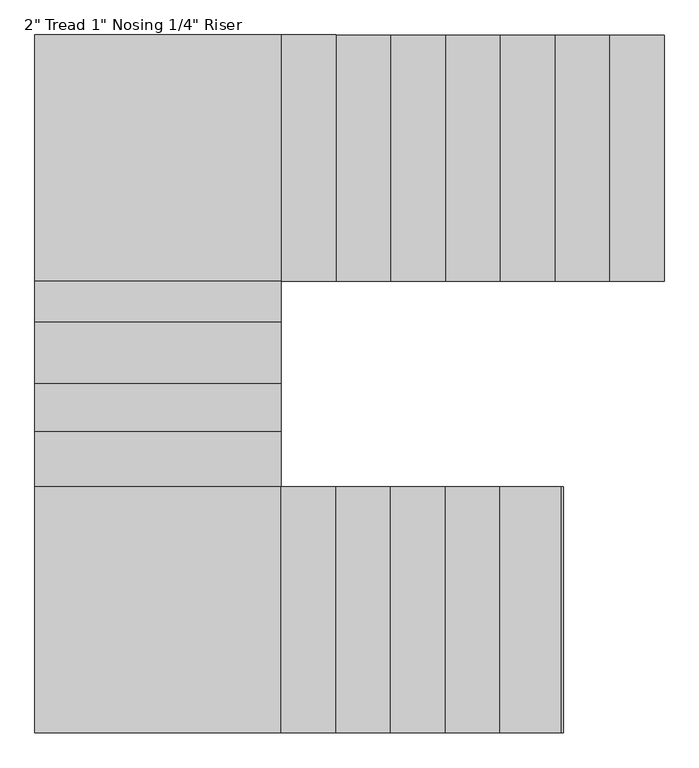
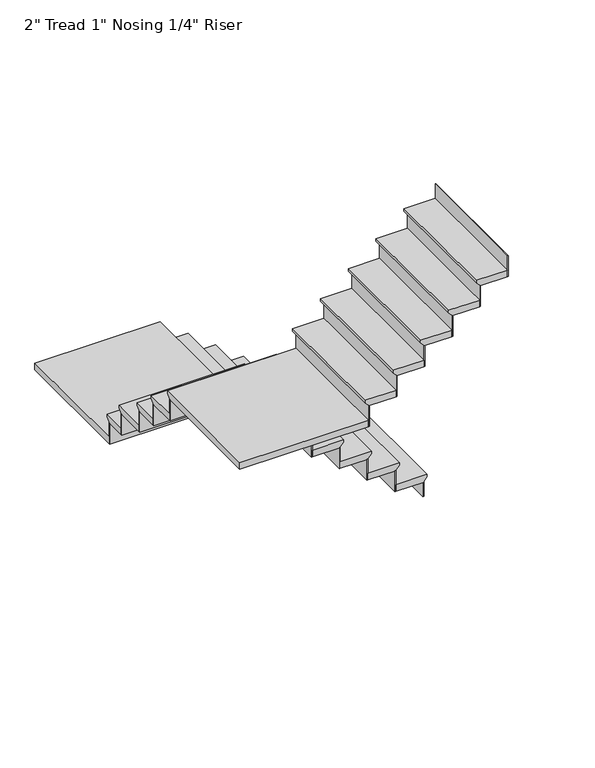
"""IFC4 building model written with IfcOpenShell, lengths in millimetres: stair flight geometry."""

from ifc_helpers import new_model, si_unit, origin, place, context, project, spatial, faceted_brep, source, transform, mapped, element, save


def stair_flight_32cec8f3(model_context):
    return source(origin(), model_context, "Body", "Brep", [
        faceted_brep([(-3603.1340247, 922.0319954, 3341.7710526), (-3603.1340247, 922.0319954, 3360.8210526), (-3603.1340247, 7.6319954, 3360.8210526), (-3603.1340247, 7.6319954, 3341.7710526), (-3628.5340247, 922.0319954, 3316.3710526), (-3628.5340247, 7.6319954, 3316.3710526), (-3831.7340247, 922.0319954, 3360.8210526), (-3831.7340247, 7.6319954, 3360.8210526), (-3628.5340247, 7.6319954, 3310.0210526), (-3831.7340247, 7.6319954, 3310.0210526), (-3831.7340247, 922.0319954, 3310.0210526), (-3628.5340247, 922.0319954, 3310.0210526)], [[[0, 1, 2, 3]], [[4, 0, 3, 5]], [[2, 1, 6, 7]], [[8, 9, 10, 11]], [[2, 7, 9, 8, 5, 3]], [[8, 11, 4, 5]], [[6, 1, 0, 4, 11, 10]], [[7, 6, 10, 9]]]),
        faceted_brep([(-3628.5340247, 922.0319954, 3310.0210526), (-3628.5340247, 922.0319954, 3200.4), (-3634.8840247, 922.0319954, 3200.4), (-3634.8840247, 922.0319954, 3310.0210526), (-3628.5340247, 7.6319954, 3310.0210526), (-3634.8840247, 7.6319954, 3310.0210526), (-3634.8840247, 7.6319954, 3200.4), (-3628.5340247, 7.6319954, 3200.4)], [[[0, 1, 2, 3]], [[4, 5, 6, 7]], [[1, 0, 4, 7]], [[2, 1, 7, 6]], [[3, 2, 6, 5]], [[0, 3, 5, 4]]]),
        faceted_brep([(-3831.7340247, 922.0319954, 3470.4421053), (-3831.7340247, 922.0319954, 3310.0210526), (-3838.0840247, 922.0319954, 3310.0210526), (-3838.0840247, 922.0319954, 3470.4421053), (-3831.7340247, 7.6319954, 3470.4421053), (-3838.0840247, 7.6319954, 3470.4421053), (-3838.0840247, 7.6319954, 3310.0210526), (-3831.7340247, 7.6319954, 3310.0210526)], [[[0, 1, 2, 3]], [[4, 5, 6, 7]], [[1, 0, 4, 7]], [[2, 1, 7, 6]], [[3, 2, 6, 5]], [[0, 3, 5, 4]]]),
        faceted_brep([(-3806.3340247, 7.6319954, 3521.2421053), (-3806.3340247, 922.0319954, 3521.2421053), (-4034.9340247, 922.0319954, 3521.2421053), (-4034.9340247, 7.6319954, 3521.2421053), (-3831.7340247, 7.6319954, 3470.4421053), (-4034.9340247, 7.6319954, 3470.4421053), (-4034.9340247, 922.0319954, 3470.4421053), (-3831.7340247, 922.0319954, 3470.4421053), (-3831.7340247, 7.6319954, 3476.7921053), (-3806.3340247, 7.6319954, 3502.1921053), (-3831.7340247, 922.0319954, 3476.7921053), (-3806.3340247, 922.0319954, 3502.1921053)], [[[0, 1, 2, 3]], [[4, 5, 6, 7]], [[0, 3, 5, 4, 8, 9]], [[4, 7, 10, 8]], [[2, 1, 11, 10, 7, 6]], [[3, 2, 6, 5]], [[11, 1, 0, 9]], [[10, 11, 9, 8]]]),
        faceted_brep([(-4034.9340247, 922.0319954, 3630.8631579), (-4034.9340247, 922.0319954, 3470.4421053), (-4041.2840247, 922.0319954, 3470.4421053), (-4041.2840247, 922.0319954, 3630.8631579), (-4034.9340247, 7.6319954, 3630.8631579), (-4041.2840247, 7.6319954, 3630.8631579), (-4041.2840247, 7.6319954, 3470.4421053), (-4034.9340247, 7.6319954, 3470.4421053)], [[[0, 1, 2, 3]], [[4, 5, 6, 7]], [[1, 0, 4, 7]], [[2, 1, 7, 6]], [[3, 2, 6, 5]], [[0, 3, 5, 4]]]),
        faceted_brep([(-4009.5340247, 7.6319954, 3681.6631579), (-4009.5340247, 922.0319954, 3681.6631579), (-4238.1340247, 922.0319954, 3681.6631579), (-4238.1340247, 7.6319954, 3681.6631579), (-4034.9340247, 7.6319954, 3630.8631579), (-4238.1340247, 7.6319954, 3630.8631579), (-4238.1340247, 922.0319954, 3630.8631579), (-4034.9340247, 922.0319954, 3630.8631579), (-4034.9340247, 7.6319954, 3637.2131579), (-4009.5340247, 7.6319954, 3662.6131579), (-4034.9340247, 922.0319954, 3637.2131579), (-4009.5340247, 922.0319954, 3662.6131579)], [[[0, 1, 2, 3]], [[4, 5, 6, 7]], [[0, 3, 5, 4, 8, 9]], [[4, 7, 10, 8]], [[2, 1, 11, 10, 7, 6]], [[3, 2, 6, 5]], [[11, 1, 0, 9]], [[10, 11, 9, 8]]]),
        faceted_brep([(-4238.1340247, 922.0319954, 3791.2842105), (-4238.1340247, 922.0319954, 3630.8631579), (-4244.4840247, 922.0319954, 3630.8631579), (-4244.4840247, 922.0319954, 3791.2842105), (-4238.1340247, 7.6319954, 3791.2842105), (-4244.4840247, 7.6319954, 3791.2842105), (-4244.4840247, 7.6319954, 3630.8631579), (-4238.1340247, 7.6319954, 3630.8631579)], [[[0, 1, 2, 3]], [[4, 5, 6, 7]], [[1, 0, 4, 7]], [[2, 1, 7, 6]], [[3, 2, 6, 5]], [[0, 3, 5, 4]]]),
        faceted_brep([(-4212.7340247, 7.6319954, 3842.0842105), (-4212.7340247, 922.0319954, 3842.0842105), (-4441.3340247, 922.0319954, 3842.0842105), (-4441.3340247, 7.6319954, 3842.0842105), (-4238.1340247, 7.6319954, 3791.2842105), (-4441.3340247, 7.6319954, 3791.2842105), (-4441.3340247, 922.0319954, 3791.2842105), (-4238.1340247, 922.0319954, 3791.2842105), (-4238.1340247, 7.6319954, 3797.6342105), (-4212.7340247, 7.6319954, 3823.0342105), (-4238.1340247, 922.0319954, 3797.6342105), (-4212.7340247, 922.0319954, 3823.0342105)], [[[0, 1, 2, 3]], [[4, 5, 6, 7]], [[0, 3, 5, 4, 8, 9]], [[4, 7, 10, 8]], [[2, 1, 11, 10, 7, 6]], [[3, 2, 6, 5]], [[11, 1, 0, 9]], [[10, 11, 9, 8]]]),
        faceted_brep([(-4441.3340247, 922.0319954, 3951.7052632), (-4441.3340247, 922.0319954, 3791.2842105), (-4447.6840247, 922.0319954, 3791.2842105), (-4447.6840247, 922.0319954, 3951.7052632), (-4441.3340247, 7.6319954, 3951.7052632), (-4447.6840247, 7.6319954, 3951.7052632), (-4447.6840247, 7.6319954, 3791.2842105), (-4441.3340247, 7.6319954, 3791.2842105)], [[[0, 1, 2, 3]], [[4, 5, 6, 7]], [[1, 0, 4, 7]], [[2, 1, 7, 6]], [[3, 2, 6, 5]], [[0, 3, 5, 4]]]),
        faceted_brep([(-4415.9340247, 7.6319954, 4002.5052632), (-4415.9340247, 922.0319954, 4002.5052632), (-4644.5340247, 922.0319954, 4002.5052632), (-4644.5340247, 7.6319954, 4002.5052632), (-4441.3340247, 7.6319954, 3951.7052632), (-4644.5340247, 7.6319954, 3951.7052632), (-4644.5340247, 922.0319954, 3951.7052632), (-4441.3340247, 922.0319954, 3951.7052632), (-4441.3340247, 7.6319954, 3958.0552632), (-4415.9340247, 7.6319954, 3983.4552632), (-4441.3340247, 922.0319954, 3958.0552632), (-4415.9340247, 922.0319954, 3983.4552632)], [[[0, 1, 2, 3]], [[4, 5, 6, 7]], [[0, 3, 5, 4, 8, 9]], [[4, 7, 10, 8]], [[2, 1, 11, 10, 7, 6]], [[3, 2, 6, 5]], [[11, 1, 0, 9]], [[10, 11, 9, 8]]]),
        faceted_brep([(-4644.5340247, 922.0319954, 4112.1263158), (-4644.5340247, 922.0319954, 3951.7052632), (-4650.8840247, 922.0319954, 3951.7052632), (-4650.8840247, 922.0319954, 4112.1263158), (-4644.5340247, 7.6319954, 4112.1263158), (-4650.8840247, 7.6319954, 4112.1263158), (-4650.8840247, 7.6319954, 3951.7052632), (-4644.5340247, 7.6319954, 3951.7052632)], [[[0, 1, 2, 3]], [[4, 5, 6, 7]], [[1, 0, 4, 7]], [[2, 1, 7, 6]], [[3, 2, 6, 5]], [[0, 3, 5, 4]]]),
        faceted_brep([(-4619.1340247, 7.6319954, 4162.9263158), (-4619.1340247, 922.0319954, 4162.9263158), (-4847.7340247, 922.0319954, 4162.9263158), (-4847.7340247, 7.6319954, 4162.9263158), (-4644.5340247, 7.6319954, 4112.1263158), (-4847.7340247, 7.6319954, 4112.1263158), (-4847.7340247, 922.0319954, 4112.1263158), (-4644.5340247, 922.0319954, 4112.1263158), (-4644.5340247, 7.6319954, 4118.4763158), (-4619.1340247, 7.6319954, 4143.8763158), (-4644.5340247, 922.0319954, 4118.4763158), (-4619.1340247, 922.0319954, 4143.8763158)], [[[0, 1, 2, 3]], [[4, 5, 6, 7]], [[0, 3, 5, 4, 8, 9]], [[4, 7, 10, 8]], [[2, 1, 11, 10, 7, 6]], [[3, 2, 6, 5]], [[11, 1, 0, 9]], [[10, 11, 9, 8]]]),
        faceted_brep([(-4847.7340247, 922.0319954, 4272.5473684), (-4847.7340247, 922.0319954, 4112.1263158), (-4854.0840247, 922.0319954, 4112.1263158), (-4854.0840247, 922.0319954, 4272.5473684), (-4847.7340247, 7.6319954, 4272.5473684), (-4854.0840247, 7.6319954, 4272.5473684), (-4854.0840247, 7.6319954, 4112.1263158), (-4847.7340247, 7.6319954, 4112.1263158)], [[[0, 1, 2, 3]], [[4, 5, 6, 7]], [[1, 0, 4, 7]], [[2, 1, 7, 6]], [[3, 2, 6, 5]], [[0, 3, 5, 4]]]),
        faceted_brep([(-4822.3340247, 7.6319954, 4323.3473684), (-4822.3340247, 922.0319954, 4323.3473684), (-5050.9340247, 922.0319954, 4323.3473684), (-5050.9340247, 7.6319954, 4323.3473684), (-4847.7340247, 7.6319954, 4272.5473684), (-5050.9340247, 7.6319954, 4272.5473684), (-5050.9340247, 922.0319954, 4272.5473684), (-4847.7340247, 922.0319954, 4272.5473684), (-4847.7340247, 7.6319954, 4278.8973684), (-4822.3340247, 7.6319954, 4304.2973684), (-4847.7340247, 922.0319954, 4278.8973684), (-4822.3340247, 922.0319954, 4304.2973684)], [[[0, 1, 2, 3]], [[4, 5, 6, 7]], [[0, 3, 5, 4, 8, 9]], [[4, 7, 10, 8]], [[2, 1, 11, 10, 7, 6]], [[3, 2, 6, 5]], [[11, 1, 0, 9]], [[10, 11, 9, 8]]]),
        faceted_brep([(-5050.9340247, 922.0319954, 4432.9684211), (-5050.9340247, 922.0319954, 4272.5473684), (-5057.2840247, 922.0319954, 4272.5473684), (-5057.2840247, 922.0319954, 4432.9684211), (-5050.9340247, 7.6319954, 4432.9684211), (-5057.2840247, 7.6319954, 4432.9684211), (-5057.2840247, 7.6319954, 4272.5473684), (-5050.9340247, 7.6319954, 4272.5473684)], [[[0, 1, 2, 3]], [[4, 5, 6, 7]], [[1, 0, 4, 7]], [[2, 1, 7, 6]], [[3, 2, 6, 5]], [[0, 3, 5, 4]]]),
        faceted_brep([(-5939.9340247, 922.0319954, 4483.7684211), (-5939.9340247, -17.7680046, 4483.7684211), (-5025.5340247, -17.7680046, 4483.7684211), (-5025.5340247, 922.0319954, 4483.7684211), (-5025.5340247, 7.6319954, 4432.9684211), (-5025.5340247, -17.7680046, 4432.9684211), (-5939.9340247, -17.7680046, 4432.9684211), (-5939.9340247, 922.0319954, 4432.9684211), (-5050.9340247, 922.0319954, 4432.9684211), (-5050.9340247, 7.6319954, 4432.9684211), (-5025.5340247, 7.6319954, 4464.7184211), (-5025.5340247, 922.0319954, 4464.7184211), (-5050.9340247, 7.6319954, 4439.3184211), (-5050.9340247, 922.0319954, 4439.3184211)], [[[0, 1, 2, 3]], [[4, 5, 6, 7, 8, 9]], [[3, 2, 5, 4, 10, 11]], [[4, 9, 12, 10]], [[9, 8, 13, 12]], [[0, 3, 11, 13, 8, 7]], [[1, 0, 7, 6]], [[2, 1, 6, 5]], [[13, 11, 10, 12]]]),
        faceted_brep([(-5939.9340247, -17.7680046, 4593.3894737), (-5939.9340247, -17.7680046, 4432.9684211), (-5939.9340247, -24.1180046, 4432.9684211), (-5939.9340247, -24.1180046, 4593.3894737), (-5025.5340247, -17.7680046, 4593.3894737), (-5025.5340247, -24.1180046, 4593.3894737), (-5025.5340247, -24.1180046, 4432.9684211), (-5025.5340247, -17.7680046, 4432.9684211)], [[[0, 1, 2, 3]], [[4, 5, 6, 7]], [[1, 0, 4, 7]], [[2, 1, 7, 6]], [[3, 2, 6, 5]], [[0, 3, 5, 4]]]),
        faceted_brep([(-5025.5340247, 7.6319954, 4644.1894737), (-5939.9340247, 7.6319954, 4644.1894737), (-5939.9340247, -170.1680046, 4644.1894737), (-5025.5340247, -170.1680046, 4644.1894737), (-5025.5340247, -17.7680046, 4593.3894737), (-5025.5340247, -170.1680046, 4593.3894737), (-5939.9340247, -170.1680046, 4593.3894737), (-5939.9340247, -17.7680046, 4593.3894737), (-5025.5340247, -17.7680046, 4599.7394737), (-5025.5340247, 7.6319954, 4625.1394737), (-5939.9340247, -17.7680046, 4599.7394737), (-5939.9340247, 7.6319954, 4625.1394737)], [[[0, 1, 2, 3]], [[4, 5, 6, 7]], [[0, 3, 5, 4, 8, 9]], [[4, 7, 10, 8]], [[2, 1, 11, 10, 7, 6]], [[3, 2, 6, 5]], [[11, 1, 0, 9]], [[10, 11, 9, 8]]]),
        faceted_brep([(-5939.9340247, -170.1680046, 4753.8105263), (-5939.9340247, -170.1680046, 4593.3894737), (-5939.9340247, -176.5180046, 4593.3894737), (-5939.9340247, -176.5180046, 4753.8105263), (-5025.5340247, -170.1680046, 4753.8105263), (-5025.5340247, -176.5180046, 4753.8105263), (-5025.5340247, -176.5180046, 4593.3894737), (-5025.5340247, -170.1680046, 4593.3894737)], [[[0, 1, 2, 3]], [[4, 5, 6, 7]], [[1, 0, 4, 7]], [[2, 1, 7, 6]], [[3, 2, 6, 5]], [[0, 3, 5, 4]]]),
        faceted_brep([(-5025.5340247, -144.7680046, 4804.6105263), (-5939.9340247, -144.7680046, 4804.6105263), (-5939.9340247, -398.7680046, 4804.6105263), (-5025.5340247, -398.7680046, 4804.6105263), (-5025.5340247, -170.1680046, 4753.8105263), (-5025.5340247, -398.7680046, 4753.8105263), (-5939.9340247, -398.7680046, 4753.8105263), (-5939.9340247, -170.1680046, 4753.8105263), (-5025.5340247, -170.1680046, 4760.1605263), (-5025.5340247, -144.7680046, 4785.5605263), (-5939.9340247, -170.1680046, 4760.1605263), (-5939.9340247, -144.7680046, 4785.5605263)], [[[0, 1, 2, 3]], [[4, 5, 6, 7]], [[0, 3, 5, 4, 8, 9]], [[4, 7, 10, 8]], [[2, 1, 11, 10, 7, 6]], [[3, 2, 6, 5]], [[11, 1, 0, 9]], [[10, 11, 9, 8]]]),
        faceted_brep([(-5939.9340247, -398.7680046, 4914.2315789), (-5939.9340247, -398.7680046, 4753.8105263), (-5939.9340247, -405.1180046, 4753.8105263), (-5939.9340247, -405.1180046, 4914.2315789), (-5025.5340247, -398.7680046, 4914.2315789), (-5025.5340247, -405.1180046, 4914.2315789), (-5025.5340247, -405.1180046, 4753.8105263), (-5025.5340247, -398.7680046, 4753.8105263)], [[[0, 1, 2, 3]], [[4, 5, 6, 7]], [[1, 0, 4, 7]], [[2, 1, 7, 6]], [[3, 2, 6, 5]], [[0, 3, 5, 4]]]),
        faceted_brep([(-5025.5340247, -373.3680046, 4965.0315789), (-5939.9340247, -373.3680046, 4965.0315789), (-5939.9340247, -576.5680046, 4965.0315789), (-5025.5340247, -576.5680046, 4965.0315789), (-5025.5340247, -398.7680046, 4914.2315789), (-5025.5340247, -576.5680046, 4914.2315789), (-5939.9340247, -576.5680046, 4914.2315789), (-5939.9340247, -398.7680046, 4914.2315789), (-5025.5340247, -398.7680046, 4920.5815789), (-5025.5340247, -373.3680046, 4945.9815789), (-5939.9340247, -398.7680046, 4920.5815789), (-5939.9340247, -373.3680046, 4945.9815789)], [[[0, 1, 2, 3]], [[4, 5, 6, 7]], [[0, 3, 5, 4, 8, 9]], [[4, 7, 10, 8]], [[2, 1, 11, 10, 7, 6]], [[3, 2, 6, 5]], [[11, 1, 0, 9]], [[10, 11, 9, 8]]]),
        faceted_brep([(-5939.9340247, -576.5680046, 5074.6526316), (-5939.9340247, -576.5680046, 4914.2315789), (-5939.9340247, -582.9180046, 4914.2315789), (-5939.9340247, -582.9180046, 5074.6526316), (-5025.5340247, -576.5680046, 5074.6526316), (-5025.5340247, -582.9180046, 5074.6526316), (-5025.5340247, -582.9180046, 4914.2315789), (-5025.5340247, -576.5680046, 4914.2315789)], [[[0, 1, 2, 3]], [[4, 5, 6, 7]], [[1, 0, 4, 7]], [[2, 1, 7, 6]], [[3, 2, 6, 5]], [[0, 3, 5, 4]]]),
        faceted_brep([(-5025.5340247, -551.1680046, 5125.4526316), (-5939.9340247, -551.1680046, 5125.4526316), (-5939.9340247, -779.7680046, 5125.4526316), (-5025.5340247, -779.7680046, 5125.4526316), (-5025.5340247, -576.5680046, 5074.6526316), (-5025.5340247, -779.7680046, 5074.6526316), (-5939.9340247, -779.7680046, 5074.6526316), (-5939.9340247, -576.5680046, 5074.6526316), (-5025.5340247, -576.5680046, 5081.0026316), (-5025.5340247, -551.1680046, 5106.4026316), (-5939.9340247, -576.5680046, 5081.0026316), (-5939.9340247, -551.1680046, 5106.4026316)], [[[0, 1, 2, 3]], [[4, 5, 6, 7]], [[0, 3, 5, 4, 8, 9]], [[4, 7, 10, 8]], [[2, 1, 11, 10, 7, 6]], [[3, 2, 6, 5]], [[11, 1, 0, 9]], [[10, 11, 9, 8]]]),
        faceted_brep([(-5939.9340247, -779.7680046, 5235.0736842), (-5939.9340247, -779.7680046, 5074.6526316), (-5939.9340247, -786.1180046, 5074.6526316), (-5939.9340247, -786.1180046, 5235.0736842), (-5025.5340247, -779.7680046, 5235.0736842), (-5025.5340247, -786.1180046, 5235.0736842), (-5025.5340247, -786.1180046, 5074.6526316), (-5025.5340247, -779.7680046, 5074.6526316)], [[[0, 1, 2, 3]], [[4, 5, 6, 7]], [[1, 0, 4, 7]], [[2, 1, 7, 6]], [[3, 2, 6, 5]], [[0, 3, 5, 4]]]),
        faceted_brep([(-5939.9340247, -1668.7680046, 5285.8736842), (-5000.1340247, -1668.7680046, 5285.8736842), (-5000.1340247, -754.3680046, 5285.8736842), (-5939.9340247, -754.3680046, 5285.8736842), (-5025.5340247, -754.3680046, 5235.0736842), (-5000.1340247, -754.3680046, 5235.0736842), (-5000.1340247, -1668.7680046, 5235.0736842), (-5939.9340247, -1668.7680046, 5235.0736842), (-5939.9340247, -779.7680046, 5235.0736842), (-5025.5340247, -779.7680046, 5235.0736842), (-5025.5340247, -754.3680046, 5266.8236842), (-5939.9340247, -754.3680046, 5266.8236842), (-5025.5340247, -779.7680046, 5241.4236842), (-5939.9340247, -779.7680046, 5241.4236842)], [[[0, 1, 2, 3]], [[4, 5, 6, 7, 8, 9]], [[3, 2, 5, 4, 10, 11]], [[4, 9, 12, 10]], [[9, 8, 13, 12]], [[0, 3, 11, 13, 8, 7]], [[1, 0, 7, 6]], [[2, 1, 6, 5]], [[13, 11, 10, 12]]]),
        faceted_brep([(-5000.1340247, -1668.7680046, 5395.4947368), (-5000.1340247, -1668.7680046, 5235.0736842), (-4993.7840247, -1668.7680046, 5235.0736842), (-4993.7840247, -1668.7680046, 5395.4947368), (-5000.1340247, -754.3680046, 5395.4947368), (-4993.7840247, -754.3680046, 5395.4947368), (-4993.7840247, -754.3680046, 5235.0736842), (-5000.1340247, -754.3680046, 5235.0736842)], [[[0, 1, 2, 3]], [[4, 5, 6, 7]], [[1, 0, 4, 7]], [[2, 1, 7, 6]], [[3, 2, 6, 5]], [[0, 3, 5, 4]]]),
        faceted_brep([(-5025.5340247, -754.3680046, 5446.2947368), (-5025.5340247, -1668.7680046, 5446.2947368), (-4796.9340247, -1668.7680046, 5446.2947368), (-4796.9340247, -754.3680046, 5446.2947368), (-5000.1340247, -754.3680046, 5395.4947368), (-4796.9340247, -754.3680046, 5395.4947368), (-4796.9340247, -1668.7680046, 5395.4947368), (-5000.1340247, -1668.7680046, 5395.4947368), (-5000.1340247, -754.3680046, 5401.8447368), (-5025.5340247, -754.3680046, 5427.2447368), (-5000.1340247, -1668.7680046, 5401.8447368), (-5025.5340247, -1668.7680046, 5427.2447368)], [[[0, 1, 2, 3]], [[4, 5, 6, 7]], [[0, 3, 5, 4, 8, 9]], [[4, 7, 10, 8]], [[2, 1, 11, 10, 7, 6]], [[3, 2, 6, 5]], [[11, 1, 0, 9]], [[10, 11, 9, 8]]]),
        faceted_brep([(-4796.9340247, -1668.7680046, 5555.9157895), (-4796.9340247, -1668.7680046, 5395.4947368), (-4790.5840247, -1668.7680046, 5395.4947368), (-4790.5840247, -1668.7680046, 5555.9157895), (-4796.9340247, -754.3680046, 5555.9157895), (-4790.5840247, -754.3680046, 5555.9157895), (-4790.5840247, -754.3680046, 5395.4947368), (-4796.9340247, -754.3680046, 5395.4947368)], [[[0, 1, 2, 3]], [[4, 5, 6, 7]], [[1, 0, 4, 7]], [[2, 1, 7, 6]], [[3, 2, 6, 5]], [[0, 3, 5, 4]]]),
        faceted_brep([(-4822.3340247, -754.3680046, 5606.7157895), (-4822.3340247, -1668.7680046, 5606.7157895), (-4593.7340247, -1668.7680046, 5606.7157895), (-4593.7340247, -754.3680046, 5606.7157895), (-4796.9340247, -754.3680046, 5555.9157895), (-4593.7340247, -754.3680046, 5555.9157895), (-4593.7340247, -1668.7680046, 5555.9157895), (-4796.9340247, -1668.7680046, 5555.9157895), (-4796.9340247, -754.3680046, 5562.2657895), (-4822.3340247, -754.3680046, 5587.6657895), (-4796.9340247, -1668.7680046, 5562.2657895), (-4822.3340247, -1668.7680046, 5587.6657895)], [[[0, 1, 2, 3]], [[4, 5, 6, 7]], [[0, 3, 5, 4, 8, 9]], [[4, 7, 10, 8]], [[2, 1, 11, 10, 7, 6]], [[3, 2, 6, 5]], [[11, 1, 0, 9]], [[10, 11, 9, 8]]]),
        faceted_brep([(-4593.7340247, -1668.7680046, 5716.3368421), (-4593.7340247, -1668.7680046, 5555.9157895), (-4587.3840247, -1668.7680046, 5555.9157895), (-4587.3840247, -1668.7680046, 5716.3368421), (-4593.7340247, -754.3680046, 5716.3368421), (-4587.3840247, -754.3680046, 5716.3368421), (-4587.3840247, -754.3680046, 5555.9157895), (-4593.7340247, -754.3680046, 5555.9157895)], [[[0, 1, 2, 3]], [[4, 5, 6, 7]], [[1, 0, 4, 7]], [[2, 1, 7, 6]], [[3, 2, 6, 5]], [[0, 3, 5, 4]]]),
        faceted_brep([(-4619.1340247, -754.3680046, 5767.1368421), (-4619.1340247, -1668.7680046, 5767.1368421), (-4390.5340247, -1668.7680046, 5767.1368421), (-4390.5340247, -754.3680046, 5767.1368421), (-4593.7340247, -754.3680046, 5716.3368421), (-4390.5340247, -754.3680046, 5716.3368421), (-4390.5340247, -1668.7680046, 5716.3368421), (-4593.7340247, -1668.7680046, 5716.3368421), (-4593.7340247, -754.3680046, 5722.6868421), (-4619.1340247, -754.3680046, 5748.0868421), (-4593.7340247, -1668.7680046, 5722.6868421), (-4619.1340247, -1668.7680046, 5748.0868421)], [[[0, 1, 2, 3]], [[4, 5, 6, 7]], [[0, 3, 5, 4, 8, 9]], [[4, 7, 10, 8]], [[2, 1, 11, 10, 7, 6]], [[3, 2, 6, 5]], [[11, 1, 0, 9]], [[10, 11, 9, 8]]]),
        faceted_brep([(-4390.5340247, -1668.7680046, 5876.7578947), (-4390.5340247, -1668.7680046, 5716.3368421), (-4384.1840247, -1668.7680046, 5716.3368421), (-4384.1840247, -1668.7680046, 5876.7578947), (-4390.5340247, -754.3680046, 5876.7578947), (-4384.1840247, -754.3680046, 5876.7578947), (-4384.1840247, -754.3680046, 5716.3368421), (-4390.5340247, -754.3680046, 5716.3368421)], [[[0, 1, 2, 3]], [[4, 5, 6, 7]], [[1, 0, 4, 7]], [[2, 1, 7, 6]], [[3, 2, 6, 5]], [[0, 3, 5, 4]]]),
        faceted_brep([(-4415.9340247, -754.3680046, 5927.5578947), (-4415.9340247, -1668.7680046, 5927.5578947), (-4187.3340247, -1668.7680046, 5927.5578947), (-4187.3340247, -754.3680046, 5927.5578947), (-4390.5340247, -754.3680046, 5876.7578947), (-4187.3340247, -754.3680046, 5876.7578947), (-4187.3340247, -1668.7680046, 5876.7578947), (-4390.5340247, -1668.7680046, 5876.7578947), (-4390.5340247, -754.3680046, 5883.1078947), (-4415.9340247, -754.3680046, 5908.5078947), (-4390.5340247, -1668.7680046, 5883.1078947), (-4415.9340247, -1668.7680046, 5908.5078947)], [[[0, 1, 2, 3]], [[4, 5, 6, 7]], [[0, 3, 5, 4, 8, 9]], [[4, 7, 10, 8]], [[2, 1, 11, 10, 7, 6]], [[3, 2, 6, 5]], [[11, 1, 0, 9]], [[10, 11, 9, 8]]]),
        faceted_brep([(-4187.3340247, -1668.7680046, 6037.1789474), (-4187.3340247, -1668.7680046, 5876.7578947), (-4180.9840247, -1668.7680046, 5876.7578947), (-4180.9840247, -1668.7680046, 6037.1789474), (-4187.3340247, -754.3680046, 6037.1789474), (-4180.9840247, -754.3680046, 6037.1789474), (-4180.9840247, -754.3680046, 5876.7578947), (-4187.3340247, -754.3680046, 5876.7578947)], [[[0, 1, 2, 3]], [[4, 5, 6, 7]], [[1, 0, 4, 7]], [[2, 1, 7, 6]], [[3, 2, 6, 5]], [[0, 3, 5, 4]]]),
        faceted_brep([(-3984.1340247, -1668.7680046, 6197.6), (-3984.1340247, -1668.7680046, 6037.1789474), (-3977.7840247, -1668.7680046, 6037.1789474), (-3977.7840247, -1668.7680046, 6197.6), (-3984.1340247, -754.3680046, 6197.6), (-3977.7840247, -754.3680046, 6197.6), (-3977.7840247, -754.3680046, 6037.1789474), (-3984.1340247, -754.3680046, 6037.1789474)], [[[0, 1, 2, 3]], [[4, 5, 6, 7]], [[1, 0, 4, 7]], [[2, 1, 7, 6]], [[3, 2, 6, 5]], [[0, 3, 5, 4]]]),
        faceted_brep([(-4212.7340247, -754.3680046, 6087.9789474), (-4212.7340247, -1668.7680046, 6087.9789474), (-3984.1340247, -1668.7680046, 6087.9789474), (-3984.1340247, -754.3680046, 6087.9789474), (-4187.3340247, -754.3680046, 6037.1789474), (-3984.1340247, -754.3680046, 6037.1789474), (-3984.1340247, -1668.7680046, 6037.1789474), (-4187.3340247, -1668.7680046, 6037.1789474), (-4187.3340247, -754.3680046, 6043.5289474), (-4212.7340247, -754.3680046, 6068.9289474), (-4187.3340247, -1668.7680046, 6043.5289474), (-4212.7340247, -1668.7680046, 6068.9289474)], [[[0, 1, 2, 3]], [[4, 5, 6, 7]], [[0, 3, 5, 4, 8, 9]], [[4, 7, 10, 8]], [[2, 1, 11, 10, 7, 6]], [[3, 2, 6, 5]], [[11, 1, 0, 9]], [[10, 11, 9, 8]]]),
    ])


if __name__ == "__main__":
    model = new_model("IFC4")
    model_context = context("Model", 3, world=origin())
    ifc_project = project(units=[si_unit("LENGTHUNIT", "METRE", prefix="MILLI")], contexts=[model_context])
    site = spatial("IfcSite", under=ifc_project)
    building = spatial("IfcBuilding", under=site)
    placement = place(None, origin())
    stair_flight_shape = stair_flight_32cec8f3(model_context)
    element("IfcStairFlight", 1, ObjectType="2\" Tread 1\" Nosing 1/4\" Riser", at=placement, inside=building, context=model_context, shape_type="MappedRepresentation", body=[
        mapped(stair_flight_shape, transform((0.0, 0.0, 0.0), x_axis=(1.0, 0.0, 0.0), y_axis=(0.0, 1.0, 0.0), z_axis=(0.0, 0.0, 1.0))),
    ])
    save(model, "model.ifc")
